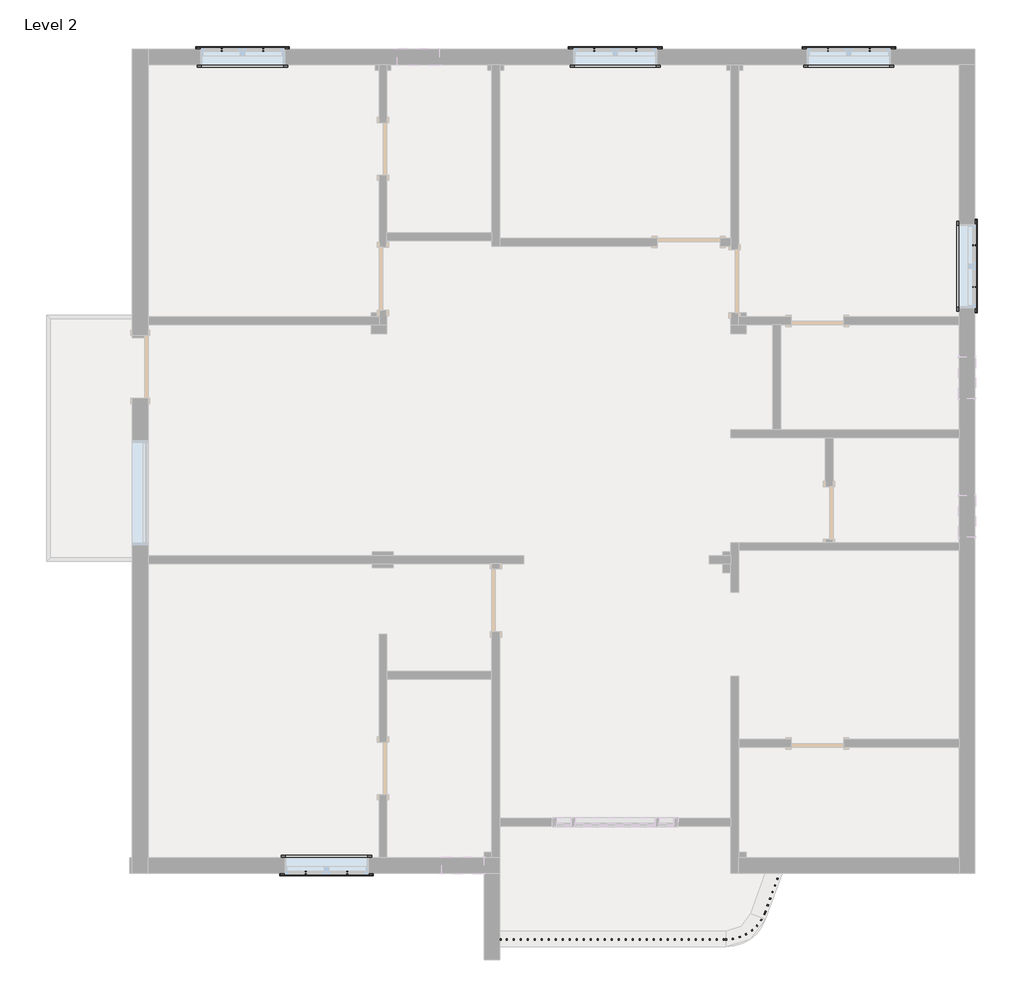
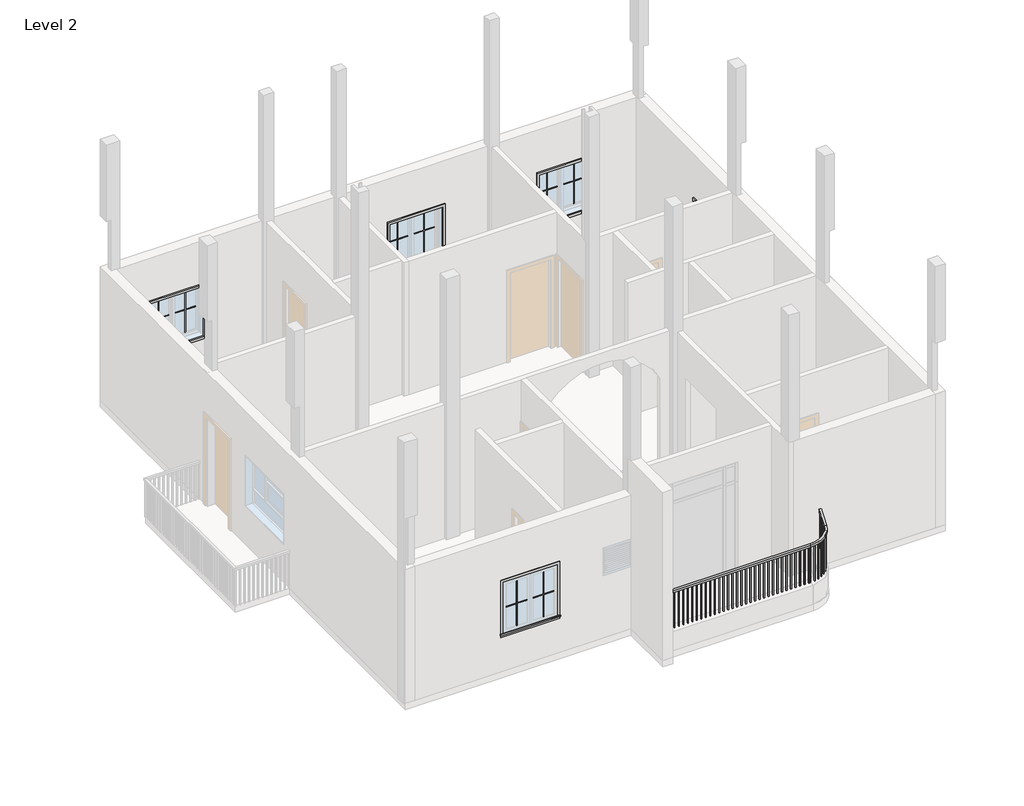
# One storey, part 4 of 4: 20 proxies, 1 railing.
"""IFC4 building model written with IfcOpenShell, lengths in millimetres."""

from ifc_helpers import new_model, si_unit, frame, origin, place, context, project, spatial, polyline, circle_curve, outline, extrude, transform, mapped, element, save
from ifc_brep_helpers import plane_surface, cylinder_surface, revolved_surface, advanced_brep
from components import muntin_pattern_2x2_muntin_pattern_2x2_4dfeb3f3, muntin_pattern_2x2_muntin_pattern_2x2_e852a7e4, trim_window_exterior_flat_with_sill_7cfdd449, trim_window_interior_flat_picture_frame_f1e0b15b

model = new_model("IFC4")

# Units and contexts
model_context = context("Model", 3, world=origin())
ifc_project = project(units=[si_unit("LENGTHUNIT", "METRE", prefix="MILLI")], contexts=[model_context])

# Site, building, storey
site = spatial("IfcSite", under=ifc_project)
building = spatial("IfcBuilding", under=site)
storey = spatial("IfcBuildingStorey", under=building, Name="Level 2", Elevation=3200.4)

# Proxies
placement = place(None, origin())
muntin_pattern_2x2_muntin_pattern_2x2_shape = muntin_pattern_2x2_muntin_pattern_2x2_4dfeb3f3(model_context)
element("IfcBuildingElementProxy", 1, Name="Muntin Pattern_2x2 : Muntin Pattern_2x2", ObjectType="Muntin Pattern_2x2 : Muntin Pattern_2x2", at=placement, inside=storey, context=model_context, shape_type="MappedRepresentation", body=[
    mapped(muntin_pattern_2x2_muntin_pattern_2x2_shape, transform((-13598.9803125, 13522.091018, 4184.65), x_axis=(1.0, 0.0, 0.0), y_axis=(0.0, 1.0, 0.0), z_axis=(0.0, 0.0, 1.0))),
])
element("IfcBuildingElementProxy", 2, Name="Muntin Pattern_2x2 : Muntin Pattern_2x2", ObjectType="Muntin Pattern_2x2 : Muntin Pattern_2x2", at=placement, inside=storey, context=model_context, shape_type="MappedRepresentation", body=[
    mapped(muntin_pattern_2x2_muntin_pattern_2x2_shape, transform((-8188.7803125, 13522.091018, 4184.65), x_axis=(1.0, 0.0, 0.0), y_axis=(0.0, 1.0, 0.0), z_axis=(0.0, 0.0, 1.0))),
])
element("IfcBuildingElementProxy", 3, Name="Muntin Pattern_2x2 : Muntin Pattern_2x2", ObjectType="Muntin Pattern_2x2 : Muntin Pattern_2x2", at=placement, inside=storey, context=model_context, shape_type="MappedRepresentation", body=[
    mapped(muntin_pattern_2x2_muntin_pattern_2x2_shape, transform((-4797.8803125, 13522.091018, 4184.65), x_axis=(1.0, 0.0, 0.0), y_axis=(0.0, 1.0, 0.0), z_axis=(0.0, 0.0, 1.0))),
])
element("IfcBuildingElementProxy", 4, Name="Muntin Pattern_2x2 : Muntin Pattern_2x2", ObjectType="Muntin Pattern_2x2 : Muntin Pattern_2x2", at=placement, inside=storey, context=model_context, shape_type="MappedRepresentation", body=[
    mapped(muntin_pattern_2x2_muntin_pattern_2x2_shape, transform((-2675.3928125, 10685.228518, 4184.65), x_axis=(0.0, -1.0, 0.0), y_axis=(1.0, 0.0, 0.0), z_axis=(0.0, 0.0, 1.0))),
])
element("IfcBuildingElementProxy", 5, Name="Muntin Pattern_2x2 : Muntin Pattern_2x2", ObjectType="Muntin Pattern_2x2 : Muntin Pattern_2x2", at=placement, inside=storey, context=model_context, shape_type="MappedRepresentation", body=[
    mapped(muntin_pattern_2x2_muntin_pattern_2x2_shape, transform((-11773.3553125, 1577.741018, 4184.65), x_axis=(-1.0, 0.0, 0.0), y_axis=(0.0, -1.0, 0.0), z_axis=(0.0, 0.0, 1.0))),
])
muntin_pattern_2x2_muntin_pattern_2x2_2_shape = muntin_pattern_2x2_muntin_pattern_2x2_e852a7e4(model_context)
element("IfcBuildingElementProxy", 6, Name="Muntin Pattern_2x2 : Muntin Pattern_2x2", ObjectType="Muntin Pattern_2x2 : Muntin Pattern_2x2", at=placement, inside=storey, context=model_context, shape_type="MappedRepresentation", body=[
    mapped(muntin_pattern_2x2_muntin_pattern_2x2_2_shape, transform((-12992.5553125, 13522.091018, 4184.65), x_axis=(-1.0, 0.0, 0.0), y_axis=(0.0, -1.0, 0.0), z_axis=(0.0, 0.0, 1.0))),
])
element("IfcBuildingElementProxy", 7, Name="Muntin Pattern_2x2 : Muntin Pattern_2x2", ObjectType="Muntin Pattern_2x2 : Muntin Pattern_2x2", at=placement, inside=storey, context=model_context, shape_type="MappedRepresentation", body=[
    mapped(muntin_pattern_2x2_muntin_pattern_2x2_2_shape, transform((-7582.3553125, 13522.091018, 4184.65), x_axis=(-1.0, 0.0, 0.0), y_axis=(0.0, -1.0, 0.0), z_axis=(0.0, 0.0, 1.0))),
])
element("IfcBuildingElementProxy", 8, Name="Muntin Pattern_2x2 : Muntin Pattern_2x2", ObjectType="Muntin Pattern_2x2 : Muntin Pattern_2x2", at=placement, inside=storey, context=model_context, shape_type="MappedRepresentation", body=[
    mapped(muntin_pattern_2x2_muntin_pattern_2x2_2_shape, transform((-4191.4553125, 13522.091018, 4184.65), x_axis=(-1.0, 0.0, 0.0), y_axis=(0.0, -1.0, 0.0), z_axis=(0.0, 0.0, 1.0))),
])
element("IfcBuildingElementProxy", 9, Name="Muntin Pattern_2x2 : Muntin Pattern_2x2", ObjectType="Muntin Pattern_2x2 : Muntin Pattern_2x2", at=placement, inside=storey, context=model_context, shape_type="MappedRepresentation", body=[
    mapped(muntin_pattern_2x2_muntin_pattern_2x2_2_shape, transform((-2675.3928125, 10078.803518, 4184.65), x_axis=(0.0, 1.0, 0.0), y_axis=(-1.0, 0.0, 0.0), z_axis=(0.0, 0.0, 1.0))),
])
element("IfcBuildingElementProxy", 10, Name="Muntin Pattern_2x2 : Muntin Pattern_2x2", ObjectType="Muntin Pattern_2x2 : Muntin Pattern_2x2", at=placement, inside=storey, context=model_context, shape_type="MappedRepresentation", body=[
    mapped(muntin_pattern_2x2_muntin_pattern_2x2_2_shape, transform((-12379.7803125, 1577.741018, 4184.65), x_axis=(1.0, 0.0, 0.0), y_axis=(0.0, 1.0, 0.0), z_axis=(0.0, 0.0, 1.0))),
])
trim_window_exterior_flat_with_sill_shape = trim_window_exterior_flat_with_sill_7cfdd449(model_context)
element("IfcBuildingElementProxy", 11, Name="Trim-Window-Exterior-Flat : with Sill", ObjectType="Trim-Window-Exterior-Flat : with Sill", at=placement, inside=storey, context=model_context, shape_type="MappedRepresentation", body=[
    mapped(trim_window_exterior_flat_with_sill_shape, transform((-13295.7678125, 13531.616018, 5334.0), x_axis=(-1.0, 0.0, 0.0), y_axis=(0.0, 0.0, 1.0), z_axis=(0.0, 1.0, 0.0))),
])
element("IfcBuildingElementProxy", 12, Name="Trim-Window-Exterior-Flat : with Sill", ObjectType="Trim-Window-Exterior-Flat : with Sill", at=placement, inside=storey, context=model_context, shape_type="MappedRepresentation", body=[
    mapped(trim_window_exterior_flat_with_sill_shape, transform((-7885.5678125, 13531.616018, 5334.0), x_axis=(-1.0, 0.0, 0.0), y_axis=(0.0, 0.0, 1.0), z_axis=(0.0, 1.0, 0.0))),
])
element("IfcBuildingElementProxy", 13, Name="Trim-Window-Exterior-Flat : with Sill", ObjectType="Trim-Window-Exterior-Flat : with Sill", at=placement, inside=storey, context=model_context, shape_type="MappedRepresentation", body=[
    mapped(trim_window_exterior_flat_with_sill_shape, transform((-4494.6678125, 13531.616018, 5334.0), x_axis=(-1.0, 0.0, 0.0), y_axis=(0.0, 0.0, 1.0), z_axis=(0.0, 1.0, 0.0))),
])
element("IfcBuildingElementProxy", 14, Name="Trim-Window-Exterior-Flat : with Sill", ObjectType="Trim-Window-Exterior-Flat : with Sill", at=placement, inside=storey, context=model_context, shape_type="MappedRepresentation", body=[
    mapped(trim_window_exterior_flat_with_sill_shape, transform((-2665.8678125, 10382.016018, 5334.0), x_axis=(0.0, 1.0, 0.0), y_axis=(0.0, 0.0, 1.0), z_axis=(1.0, 0.0, 0.0))),
])
element("IfcBuildingElementProxy", 15, Name="Trim-Window-Exterior-Flat : with Sill", ObjectType="Trim-Window-Exterior-Flat : with Sill", at=placement, inside=storey, context=model_context, shape_type="MappedRepresentation", body=[
    mapped(trim_window_exterior_flat_with_sill_shape, transform((-12076.5678125, 1568.216018, 5334.0), x_axis=(1.0, 0.0, 0.0), y_axis=(0.0, 0.0, 1.0), z_axis=(0.0, -1.0, 0.0))),
])
trim_window_interior_flat_picture_frame_shape = trim_window_interior_flat_picture_frame_f1e0b15b(model_context)
element("IfcBuildingElementProxy", 16, Name="Trim-Window-Interior-Flat : Picture Frame", ObjectType="Trim-Window-Interior-Flat : Picture Frame", at=placement, inside=storey, context=model_context, shape_type="MappedRepresentation", body=[
    mapped(trim_window_interior_flat_picture_frame_shape, transform((-13295.7678125, 13303.016018, 5334.0), x_axis=(1.0, 0.0, 0.0), y_axis=(0.0, 0.0, 1.0), z_axis=(0.0, -1.0, 0.0))),
])
element("IfcBuildingElementProxy", 17, Name="Trim-Window-Interior-Flat : Picture Frame", ObjectType="Trim-Window-Interior-Flat : Picture Frame", at=placement, inside=storey, context=model_context, shape_type="MappedRepresentation", body=[
    mapped(trim_window_interior_flat_picture_frame_shape, transform((-7885.5678125, 13303.016018, 5334.0), x_axis=(1.0, 0.0, 0.0), y_axis=(0.0, 0.0, 1.0), z_axis=(0.0, -1.0, 0.0))),
])
element("IfcBuildingElementProxy", 18, Name="Trim-Window-Interior-Flat : Picture Frame", ObjectType="Trim-Window-Interior-Flat : Picture Frame", at=placement, inside=storey, context=model_context, shape_type="MappedRepresentation", body=[
    mapped(trim_window_interior_flat_picture_frame_shape, transform((-4494.6678125, 13303.016018, 5334.0), x_axis=(1.0, 0.0, 0.0), y_axis=(0.0, 0.0, 1.0), z_axis=(0.0, -1.0, 0.0))),
])
element("IfcBuildingElementProxy", 19, Name="Trim-Window-Interior-Flat : Picture Frame", ObjectType="Trim-Window-Interior-Flat : Picture Frame", at=placement, inside=storey, context=model_context, shape_type="MappedRepresentation", body=[
    mapped(trim_window_interior_flat_picture_frame_shape, transform((-2894.4678125, 10382.016018, 5334.0), x_axis=(0.0, -1.0, 0.0), y_axis=(0.0, 0.0, 1.0), z_axis=(-1.0, 0.0, 0.0))),
])
element("IfcBuildingElementProxy", 20, Name="Trim-Window-Interior-Flat : Picture Frame", ObjectType="Trim-Window-Interior-Flat : Picture Frame", at=placement, inside=storey, context=model_context, shape_type="MappedRepresentation", body=[
    mapped(trim_window_interior_flat_picture_frame_shape, transform((-12076.5678125, 1796.816018, 5334.0), x_axis=(-1.0, 0.0, 0.0), y_axis=(0.0, 0.0, 1.0), z_axis=(0.0, 1.0, 0.0))),
])

# Railing
element("IfcRailing", 21, ObjectType="Handrail - Rectangular", at=placement, inside=storey, context=model_context, shape_type="SolidModel", body=[
    advanced_brep(
    [(-9561.9678125, 634.766018, 4572.0), (-9561.9678125, 634.766018, 4521.2), (-9561.9678125, 583.966018, 4521.2), (-9561.9678125, 583.966018, 4572.0), (-6278.443289, 634.766018, 4572.0), (-6278.443289, 634.766018, 4521.2), (-6278.443289, 583.966018, 4521.2), (-6278.443289, 583.966018, 4572.0), (-5729.4748599, 1019.1578503, 4521.2), (-5729.4748599, 1019.1578503, 4572.0), (-5681.7384748, 1001.783227, 4521.2), (-5681.7384748, 1001.783227, 4572.0), (-5487.1815204, 1684.8533296, 4572.0), (-5439.4451352, 1667.4787064, 4572.0), (-5439.4451352, 1667.4787064, 4521.2), (-5487.1815204, 1684.8533296, 4521.2)],
    [
        (0, 1),
        (1, 2),
        (2, 3),
        (3, 0),
        (0, 4),
        (4, 5),
        (5, 1),
        (5, 6),
        (6, 2),
        (6, 7),
        (7, 3),
        (7, 4),
        (8, 5, circle_curve(frame((-6278.443289, 1218.966018, 4521.2), z_axis=(0.0, 0.0, -1.0), x_axis=(0.0, -1.0, 0.0)), 584.2)),
        (4, 9, circle_curve(frame((-6278.443289, 1218.966018, 4572.0), z_axis=(0.0, 0.0, 1.0), x_axis=(0.0, -1.0, 0.0)), 584.2)),
        (9, 8),
        (10, 6, circle_curve(frame((-6278.443289, 1218.966018, 4521.2), z_axis=(0.0, 0.0, -1.0), x_axis=(0.0, -1.0, 0.0)), 635.0)),
        (8, 10),
        (11, 7, circle_curve(frame((-6278.443289, 1218.966018, 4572.0), z_axis=(0.0, 0.0, -1.0), x_axis=(0.0, -1.0, 0.0)), 635.0)),
        (10, 11),
        (11, 9),
        (12, 13),
        (13, 14),
        (14, 15),
        (15, 12),
        (9, 12),
        (15, 8),
        (14, 10),
        (13, 11),
    ],
    [
        plane_surface(frame((-9561.9678125, 609.366018, 4572.0), z_axis=(-1.0, 0.0, 0.0), x_axis=(0.0, 1.0, 0.0))),
        plane_surface(frame((-9561.9678125, 634.766018, 4572.0), z_axis=(0.0, 1.0, 0.0), x_axis=(1.0, 0.0, 0.0))),
        plane_surface(frame((-9561.9678125, 634.766018, 4521.2), z_axis=(0.0, 0.0, -1.0), x_axis=(1.0, 0.0, 0.0))),
        plane_surface(frame((-9561.9678125, 583.966018, 4521.2), z_axis=(0.0, -1.0, 0.0), x_axis=(1.0, 0.0, 0.0))),
        plane_surface(frame((-9561.9678125, 583.966018, 4572.0), z_axis=(0.0, 0.0, 1.0), x_axis=(1.0, 0.0, 0.0))),
        revolved_surface(polyline([(-6278.443289, 634.766018, 4572.0), (-6278.443289, 634.766018, 4521.2)]), (-6278.443289, 1218.966018, 4572.0), (0.0, 0.0, 1.0)),
        plane_surface(frame((-6278.443289, 1218.966018, 4521.2), z_axis=(0.0, 0.0, -1.0), x_axis=(0.0, -1.0, 0.0))),
        cylinder_surface(frame((-6278.443289, 1218.966018, 4572.0), z_axis=(0.0, 0.0, 1.0), x_axis=(0.0, -1.0, 0.0)), 635.0),
        plane_surface(frame((-6278.443289, 1218.966018, 4572.0), z_axis=(0.0, 0.0, 1.0), x_axis=(0.0, -1.0, 0.0))),
        plane_surface(frame((-5463.3133278, 1676.166018, 4572.0), z_axis=(0.3420201433256705, 0.9396926207859078, 0.0), x_axis=(0.9396926207859078, -0.3420201433256705, 0.0))),
        plane_surface(frame((-5729.4748599, 1019.1578503, 4572.0), z_axis=(-0.9396926207859078, 0.3420201433256704, 0.0), x_axis=(0.3420201433256704, 0.9396926207859078, 0.0))),
        plane_surface(frame((-5729.4748599, 1019.1578503, 4521.2), z_axis=(0.0, 0.0, -1.0), x_axis=(0.3420201433256704, 0.9396926207859078, 0.0))),
        plane_surface(frame((-5681.7384748, 1001.783227, 4521.2), z_axis=(0.9396926207859079, -0.3420201433256703, 0.0), x_axis=(0.3420201433256703, 0.9396926207859079, 0.0))),
        plane_surface(frame((-5681.7384748, 1001.783227, 4572.0), z_axis=(0.0, 0.0, 1.0), x_axis=(0.3420201433256703, 0.9396926207859079, 0.0))),
    ],
    [
        (0, [[1, 2, 3, 4]]),
        (1, [[-1, 5, 6, 7]]),
        (2, [[-2, -7, 8, 9]]),
        (3, [[-3, -9, 10, 11]]),
        (4, [[-4, -11, 12, -5]]),
        (5, [[13, -6, 14, 15]]),
        (6, [[16, -8, -13, 17]]),
        (7, [[18, -10, -16, 19]]),
        (8, [[-14, -12, -18, 20]]),
        (9, [[21, 22, 23, 24]]),
        (10, [[-15, 25, -24, 26]]),
        (11, [[-17, -26, -23, 27]]),
        (12, [[-19, -27, -22, 28]]),
        (13, [[-20, -28, -21, -25]]),
    ],
),
    extrude(outline(polyline([(-5491.4183577, 1571.0988462), (-5509.3195021, 1577.6143299), (-5502.8040184, 1595.5154743), (-5484.9028739, 1588.9999906), (-5491.4183577, 1571.0988462)])), frame((0.0, 0.0, 3657.6), z_axis=(0.0, 0.0, 1.0), x_axis=(1.0, 0.0, 0.0)), (0.0, 0.0, 1.0), 863.6),
    extrude(outline(polyline([(-5526.1676042, 1475.6260759), (-5544.0687486, 1482.1415596), (-5537.5532649, 1500.0427041), (-5519.6521205, 1493.5272203), (-5526.1676042, 1475.6260759)])), frame((0.0, 0.0, 3657.6), z_axis=(0.0, 0.0, 1.0), x_axis=(1.0, 0.0, 0.0)), (0.0, 0.0, 1.0), 863.6),
    extrude(outline(polyline([(-5560.9168508, 1380.1533056), (-5578.8179952, 1386.6687894), (-5572.3025115, 1404.5699338), (-5554.4013671, 1398.0544501), (-5560.9168508, 1380.1533056)])), frame((0.0, 0.0, 3657.6), z_axis=(0.0, 0.0, 1.0), x_axis=(1.0, 0.0, 0.0)), (0.0, 0.0, 1.0), 863.6),
    extrude(outline(polyline([(-5595.6660973, 1284.6805354), (-5613.5672418, 1291.1960191), (-5607.051758, 1309.0971635), (-5589.1506136, 1302.5816798), (-5595.6660973, 1284.6805354)])), frame((0.0, 0.0, 3657.6), z_axis=(0.0, 0.0, 1.0), x_axis=(1.0, 0.0, 0.0)), (0.0, 0.0, 1.0), 863.6),
    extrude(outline(polyline([(-5630.4153439, 1189.2077651), (-5648.3164883, 1195.7232488), (-5641.8010046, 1213.6243932), (-5623.8998602, 1207.1089095), (-5630.4153439, 1189.2077651)])), frame((0.0, 0.0, 3657.6), z_axis=(0.0, 0.0, 1.0), x_axis=(1.0, 0.0, 0.0)), (0.0, 0.0, 1.0), 863.6),
    extrude(outline(polyline([(-5665.1645905, 1093.7349948), (-5683.0657349, 1100.2504785), (-5676.5502512, 1118.151623), (-5658.6491067, 1111.6361392), (-5665.1645905, 1093.7349948)])), frame((0.0, 0.0, 3657.6), z_axis=(0.0, 0.0, 1.0), x_axis=(1.0, 0.0, 0.0)), (0.0, 0.0, 1.0), 863.6),
    extrude(outline(polyline([(-5712.9373242, 966.7567894), (-5730.452751, 974.2476053), (-5722.9619352, 991.7630322), (-5705.4465083, 984.2722163), (-5712.9373242, 966.7567894)])), frame((0.0, 0.0, 3657.6), z_axis=(0.0, 0.0, 1.0), x_axis=(1.0, 0.0, 0.0)), (0.0, 0.0, 1.0), 863.6),
    extrude(outline(polyline([(-5762.613945, 876.4363417), (-5778.6439673, 886.7291007), (-5768.3512083, 902.7591229), (-5752.3211861, 892.466364), (-5762.613945, 876.4363417)])), frame((0.0, 0.0, 3657.6), z_axis=(0.0, 0.0, 1.0), x_axis=(1.0, 0.0, 0.0)), (0.0, 0.0, 1.0), 863.6),
    extrude(outline(polyline([(-5826.5860214, 795.6086028), (-5840.6863905, 808.4180561), (-5827.8769372, 822.5184252), (-5813.7765681, 809.7089719), (-5826.5860214, 795.6086028)])), frame((0.0, 0.0, 3657.6), z_axis=(0.0, 0.0, 1.0), x_axis=(1.0, 0.0, 0.0)), (0.0, 0.0, 1.0), 863.6),
    extrude(outline(polyline([(-5903.0806608, 726.5135953), (-5914.8606056, 741.4847476), (-5899.8894533, 753.2646924), (-5888.1095085, 738.29354), (-5903.0806608, 726.5135953)])), frame((0.0, 0.0, 3657.6), z_axis=(0.0, 0.0, 1.0), x_axis=(1.0, 0.0, 0.0)), (0.0, 0.0, 1.0), 863.6),
    extrude(outline(polyline([(-5989.9779263, 671.0661861), (-5999.1109828, 687.7841339), (-5982.393035, 696.9171904), (-5973.2599785, 680.1992426), (-5989.9779263, 671.0661861)])), frame((0.0, 0.0, 3657.6), z_axis=(0.0, 0.0, 1.0), x_axis=(1.0, 0.0, 0.0)), (0.0, 0.0, 1.0), 863.6),
    extrude(outline(polyline([(-6084.8695873, 630.8030191), (-6091.1026462, 648.8044489), (-6073.1012164, 655.0375079), (-6066.8681574, 637.0360781), (-6084.8695873, 630.8030191)])), frame((0.0, 0.0, 3657.6), z_axis=(0.0, 0.0, 1.0), x_axis=(1.0, 0.0, 0.0)), (0.0, 0.0, 1.0), 863.6),
    extrude(outline(polyline([(-6185.1258601, 606.8399291), (-6188.2861815, 625.6259576), (-6169.5001529, 628.786279), (-6166.3398316, 610.0002504), (-6185.1258601, 606.8399291)])), frame((0.0, 0.0, 3657.6), z_axis=(0.0, 0.0, 1.0), x_axis=(1.0, 0.0, 0.0)), (0.0, 0.0, 1.0), 863.6),
    extrude(outline(polyline([(-6320.2928125, 599.841018), (-6320.2928125, 618.891018), (-6301.2428125, 618.891018), (-6301.2428125, 599.841018), (-6320.2928125, 599.841018)])), frame((0.0, 0.0, 3657.6), z_axis=(0.0, 0.0, 1.0), x_axis=(1.0, 0.0, 0.0)), (0.0, 0.0, 1.0), 863.6),
    extrude(outline(polyline([(-6421.8928125, 599.841018), (-6421.8928125, 618.891018), (-6402.8428125, 618.891018), (-6402.8428125, 599.841018), (-6421.8928125, 599.841018)])), frame((0.0, 0.0, 3657.6), z_axis=(0.0, 0.0, 1.0), x_axis=(1.0, 0.0, 0.0)), (0.0, 0.0, 1.0), 863.6),
    extrude(outline(polyline([(-6523.4928125, 599.841018), (-6523.4928125, 618.891018), (-6504.4428125, 618.891018), (-6504.4428125, 599.841018), (-6523.4928125, 599.841018)])), frame((0.0, 0.0, 3657.6), z_axis=(0.0, 0.0, 1.0), x_axis=(1.0, 0.0, 0.0)), (0.0, 0.0, 1.0), 863.6),
    extrude(outline(polyline([(-6625.0928125, 599.841018), (-6625.0928125, 618.891018), (-6606.0428125, 618.891018), (-6606.0428125, 599.841018), (-6625.0928125, 599.841018)])), frame((0.0, 0.0, 3657.6), z_axis=(0.0, 0.0, 1.0), x_axis=(1.0, 0.0, 0.0)), (0.0, 0.0, 1.0), 863.6),
    extrude(outline(polyline([(-6726.6928125, 599.841018), (-6726.6928125, 618.891018), (-6707.6428125, 618.891018), (-6707.6428125, 599.841018), (-6726.6928125, 599.841018)])), frame((0.0, 0.0, 3657.6), z_axis=(0.0, 0.0, 1.0), x_axis=(1.0, 0.0, 0.0)), (0.0, 0.0, 1.0), 863.6),
    extrude(outline(polyline([(-6828.2928125, 599.841018), (-6828.2928125, 618.891018), (-6809.2428125, 618.891018), (-6809.2428125, 599.841018), (-6828.2928125, 599.841018)])), frame((0.0, 0.0, 3657.6), z_axis=(0.0, 0.0, 1.0), x_axis=(1.0, 0.0, 0.0)), (0.0, 0.0, 1.0), 863.6),
    extrude(outline(polyline([(-6929.8928125, 599.841018), (-6929.8928125, 618.891018), (-6910.8428125, 618.891018), (-6910.8428125, 599.841018), (-6929.8928125, 599.841018)])), frame((0.0, 0.0, 3657.6), z_axis=(0.0, 0.0, 1.0), x_axis=(1.0, 0.0, 0.0)), (0.0, 0.0, 1.0), 863.6),
    extrude(outline(polyline([(-7031.4928125, 599.841018), (-7031.4928125, 618.891018), (-7012.4428125, 618.891018), (-7012.4428125, 599.841018), (-7031.4928125, 599.841018)])), frame((0.0, 0.0, 3657.6), z_axis=(0.0, 0.0, 1.0), x_axis=(1.0, 0.0, 0.0)), (0.0, 0.0, 1.0), 863.6),
    extrude(outline(polyline([(-7133.0928125, 599.841018), (-7133.0928125, 618.891018), (-7114.0428125, 618.891018), (-7114.0428125, 599.841018), (-7133.0928125, 599.841018)])), frame((0.0, 0.0, 3657.6), z_axis=(0.0, 0.0, 1.0), x_axis=(1.0, 0.0, 0.0)), (0.0, 0.0, 1.0), 863.6),
    extrude(outline(polyline([(-7234.6928125, 599.841018), (-7234.6928125, 618.891018), (-7215.6428125, 618.891018), (-7215.6428125, 599.841018), (-7234.6928125, 599.841018)])), frame((0.0, 0.0, 3657.6), z_axis=(0.0, 0.0, 1.0), x_axis=(1.0, 0.0, 0.0)), (0.0, 0.0, 1.0), 863.6),
    extrude(outline(polyline([(-7336.2928125, 599.841018), (-7336.2928125, 618.891018), (-7317.2428125, 618.891018), (-7317.2428125, 599.841018), (-7336.2928125, 599.841018)])), frame((0.0, 0.0, 3657.6), z_axis=(0.0, 0.0, 1.0), x_axis=(1.0, 0.0, 0.0)), (0.0, 0.0, 1.0), 863.6),
    extrude(outline(polyline([(-7437.8928125, 599.841018), (-7437.8928125, 618.891018), (-7418.8428125, 618.891018), (-7418.8428125, 599.841018), (-7437.8928125, 599.841018)])), frame((0.0, 0.0, 3657.6), z_axis=(0.0, 0.0, 1.0), x_axis=(1.0, 0.0, 0.0)), (0.0, 0.0, 1.0), 863.6),
    extrude(outline(polyline([(-7539.4928125, 599.841018), (-7539.4928125, 618.891018), (-7520.4428125, 618.891018), (-7520.4428125, 599.841018), (-7539.4928125, 599.841018)])), frame((0.0, 0.0, 3657.6), z_axis=(0.0, 0.0, 1.0), x_axis=(1.0, 0.0, 0.0)), (0.0, 0.0, 1.0), 863.6),
    extrude(outline(polyline([(-7641.0928125, 599.841018), (-7641.0928125, 618.891018), (-7622.0428125, 618.891018), (-7622.0428125, 599.841018), (-7641.0928125, 599.841018)])), frame((0.0, 0.0, 3657.6), z_axis=(0.0, 0.0, 1.0), x_axis=(1.0, 0.0, 0.0)), (0.0, 0.0, 1.0), 863.6),
    extrude(outline(polyline([(-7742.6928125, 599.841018), (-7742.6928125, 618.891018), (-7723.6428125, 618.891018), (-7723.6428125, 599.841018), (-7742.6928125, 599.841018)])), frame((0.0, 0.0, 3657.6), z_axis=(0.0, 0.0, 1.0), x_axis=(1.0, 0.0, 0.0)), (0.0, 0.0, 1.0), 863.6),
    extrude(outline(polyline([(-7844.2928125, 599.841018), (-7844.2928125, 618.891018), (-7825.2428125, 618.891018), (-7825.2428125, 599.841018), (-7844.2928125, 599.841018)])), frame((0.0, 0.0, 3657.6), z_axis=(0.0, 0.0, 1.0), x_axis=(1.0, 0.0, 0.0)), (0.0, 0.0, 1.0), 863.6),
    extrude(outline(polyline([(-7945.8928125, 599.841018), (-7945.8928125, 618.891018), (-7926.8428125, 618.891018), (-7926.8428125, 599.841018), (-7945.8928125, 599.841018)])), frame((0.0, 0.0, 3657.6), z_axis=(0.0, 0.0, 1.0), x_axis=(1.0, 0.0, 0.0)), (0.0, 0.0, 1.0), 863.6),
    extrude(outline(polyline([(-8047.4928125, 599.841018), (-8047.4928125, 618.891018), (-8028.4428125, 618.891018), (-8028.4428125, 599.841018), (-8047.4928125, 599.841018)])), frame((0.0, 0.0, 3657.6), z_axis=(0.0, 0.0, 1.0), x_axis=(1.0, 0.0, 0.0)), (0.0, 0.0, 1.0), 863.6),
    extrude(outline(polyline([(-8149.0928125, 599.841018), (-8149.0928125, 618.891018), (-8130.0428125, 618.891018), (-8130.0428125, 599.841018), (-8149.0928125, 599.841018)])), frame((0.0, 0.0, 3657.6), z_axis=(0.0, 0.0, 1.0), x_axis=(1.0, 0.0, 0.0)), (0.0, 0.0, 1.0), 863.6),
    extrude(outline(polyline([(-8250.6928125, 599.841018), (-8250.6928125, 618.891018), (-8231.6428125, 618.891018), (-8231.6428125, 599.841018), (-8250.6928125, 599.841018)])), frame((0.0, 0.0, 3657.6), z_axis=(0.0, 0.0, 1.0), x_axis=(1.0, 0.0, 0.0)), (0.0, 0.0, 1.0), 863.6),
    extrude(outline(polyline([(-8352.2928125, 599.841018), (-8352.2928125, 618.891018), (-8333.2428125, 618.891018), (-8333.2428125, 599.841018), (-8352.2928125, 599.841018)])), frame((0.0, 0.0, 3657.6), z_axis=(0.0, 0.0, 1.0), x_axis=(1.0, 0.0, 0.0)), (0.0, 0.0, 1.0), 863.6),
    extrude(outline(polyline([(-8453.8928125, 599.841018), (-8453.8928125, 618.891018), (-8434.8428125, 618.891018), (-8434.8428125, 599.841018), (-8453.8928125, 599.841018)])), frame((0.0, 0.0, 3657.6), z_axis=(0.0, 0.0, 1.0), x_axis=(1.0, 0.0, 0.0)), (0.0, 0.0, 1.0), 863.6),
    extrude(outline(polyline([(-8555.4928125, 599.841018), (-8555.4928125, 618.891018), (-8536.4428125, 618.891018), (-8536.4428125, 599.841018), (-8555.4928125, 599.841018)])), frame((0.0, 0.0, 3657.6), z_axis=(0.0, 0.0, 1.0), x_axis=(1.0, 0.0, 0.0)), (0.0, 0.0, 1.0), 863.6),
    extrude(outline(polyline([(-8657.0928125, 599.841018), (-8657.0928125, 618.891018), (-8638.0428125, 618.891018), (-8638.0428125, 599.841018), (-8657.0928125, 599.841018)])), frame((0.0, 0.0, 3657.6), z_axis=(0.0, 0.0, 1.0), x_axis=(1.0, 0.0, 0.0)), (0.0, 0.0, 1.0), 863.6),
    extrude(outline(polyline([(-8758.6928125, 599.841018), (-8758.6928125, 618.891018), (-8739.6428125, 618.891018), (-8739.6428125, 599.841018), (-8758.6928125, 599.841018)])), frame((0.0, 0.0, 3657.6), z_axis=(0.0, 0.0, 1.0), x_axis=(1.0, 0.0, 0.0)), (0.0, 0.0, 1.0), 863.6),
    extrude(outline(polyline([(-8860.2928125, 599.841018), (-8860.2928125, 618.891018), (-8841.2428125, 618.891018), (-8841.2428125, 599.841018), (-8860.2928125, 599.841018)])), frame((0.0, 0.0, 3657.6), z_axis=(0.0, 0.0, 1.0), x_axis=(1.0, 0.0, 0.0)), (0.0, 0.0, 1.0), 863.6),
    extrude(outline(polyline([(-8961.8928125, 599.841018), (-8961.8928125, 618.891018), (-8942.8428125, 618.891018), (-8942.8428125, 599.841018), (-8961.8928125, 599.841018)])), frame((0.0, 0.0, 3657.6), z_axis=(0.0, 0.0, 1.0), x_axis=(1.0, 0.0, 0.0)), (0.0, 0.0, 1.0), 863.6),
    extrude(outline(polyline([(-9063.4928125, 599.841018), (-9063.4928125, 618.891018), (-9044.4428125, 618.891018), (-9044.4428125, 599.841018), (-9063.4928125, 599.841018)])), frame((0.0, 0.0, 3657.6), z_axis=(0.0, 0.0, 1.0), x_axis=(1.0, 0.0, 0.0)), (0.0, 0.0, 1.0), 863.6),
    extrude(outline(polyline([(-9165.0928125, 599.841018), (-9165.0928125, 618.891018), (-9146.0428125, 618.891018), (-9146.0428125, 599.841018), (-9165.0928125, 599.841018)])), frame((0.0, 0.0, 3657.6), z_axis=(0.0, 0.0, 1.0), x_axis=(1.0, 0.0, 0.0)), (0.0, 0.0, 1.0), 863.6),
    extrude(outline(polyline([(-9266.6928125, 599.841018), (-9266.6928125, 618.891018), (-9247.6428125, 618.891018), (-9247.6428125, 599.841018), (-9266.6928125, 599.841018)])), frame((0.0, 0.0, 3657.6), z_axis=(0.0, 0.0, 1.0), x_axis=(1.0, 0.0, 0.0)), (0.0, 0.0, 1.0), 863.6),
    extrude(outline(polyline([(-9368.2928125, 599.841018), (-9368.2928125, 618.891018), (-9349.2428125, 618.891018), (-9349.2428125, 599.841018), (-9368.2928125, 599.841018)])), frame((0.0, 0.0, 3657.6), z_axis=(0.0, 0.0, 1.0), x_axis=(1.0, 0.0, 0.0)), (0.0, 0.0, 1.0), 863.6),
    extrude(outline(polyline([(-9469.8928125, 599.841018), (-9469.8928125, 618.891018), (-9450.8428125, 618.891018), (-9450.8428125, 599.841018), (-9469.8928125, 599.841018)])), frame((0.0, 0.0, 3657.6), z_axis=(0.0, 0.0, 1.0), x_axis=(1.0, 0.0, 0.0)), (0.0, 0.0, 1.0), 863.6),
    extrude(outline(polyline([(-5699.913837, 998.2622245), (-5717.8149815, 1004.7777083), (-5711.2994977, 1022.6788527), (-5693.3983533, 1016.163369), (-5699.913837, 998.2622245)])), frame((0.0, 0.0, 3657.6), z_axis=(0.0, 0.0, 1.0), x_axis=(1.0, 0.0, 0.0)), (0.0, 0.0, 1.0), 863.6),
    extrude(outline(polyline([(-6287.968289, 599.841018), (-6287.968289, 618.891018), (-6268.918289, 618.891018), (-6268.918289, 599.841018), (-6287.968289, 599.841018)])), frame((0.0, 0.0, 3657.6), z_axis=(0.0, 0.0, 1.0), x_axis=(1.0, 0.0, 0.0)), (0.0, 0.0, 1.0), 863.6),
    extrude(outline(polyline([(-5460.8782393, 1655.0071317), (-5478.7793837, 1661.5226154), (-5472.2639, 1679.4237599), (-5454.3627556, 1672.9082761), (-5460.8782393, 1655.0071317)])), frame((0.0, 0.0, 3657.6), z_axis=(0.0, 0.0, 1.0), x_axis=(1.0, 0.0, 0.0)), (0.0, 0.0, 1.0), 863.6),
    extrude(outline(polyline([(-9561.9678125, 599.841018), (-9561.9678125, 618.891018), (-9542.9178125, 618.891018), (-9542.9178125, 599.841018), (-9561.9678125, 599.841018)])), frame((0.0, 0.0, 3657.6), z_axis=(0.0, 0.0, 1.0), x_axis=(1.0, 0.0, 0.0)), (0.0, 0.0, 1.0), 863.6),
])

save(model, "model.ifc")

# Revit data of these elements
# Type "Muntin Pattern_2x2 : Muntin Pattern_2x2"
#   Width [instance default] = 4' - 0"
#   Thickness = 0' - 0 1/2"
#   Height [instance default] = 4' - 0"
#   Distance = 0' - 0 3/4"
#   Interior Material [instance default] = none
#   Exterior Material [instance default] = none
#   Default Elevation = 0
# Type "Trim-Window-Exterior-Flat : with Sill"
#   Trim Width = 0' - 2 1/4"
#   Trim Thickness_Picture Frame = 0' - 1 1/4"
#   Trim Thickness_with Sill = 0' - 0 3/4"
#   Sill Thickness = 0' - 1 1/4"
#   Opening Width [instance default] = 2' - 0"
#   Opening Height [instance default] = 3' - 0"
#   Default Elevation = 4' - 0"
#   Sill = yes
#   Picture Frame = no
#   Trim Material [instance default] = none
# Type "Trim-Window-Interior-Flat : Picture Frame"
#   Trim Thickness_Picture Frame = 0' - 1 1/4"
#   Trim Width = 0' - 2 1/4"
#   Trim Thickness_with Sill = 0' - 0 3/4"
#   Sill Thickness = 0' - 1 1/4"
#   Opening Width [instance default] = 2' - 0"
#   Opening Height [instance default] = 3' - 0"
#   Default Elevation = 4' - 0"
#   Sill = no
#   Picture Frame = yes
#   Trim Material [instance default] = none
# Type "Handrail - Rectangular"
#   Assembly Code = "C2010400"
#   built-in parameter 1008612 = 0.0416667 (stored number, unit not read)
#   built-in parameter 1008611 = 0.0416667 (stored number, unit not read)
#   built-in parameter 1008609 = 0.333333 (stored number, unit not read)
#   built-in parameter 1008604 = 0.166667 (stored number, unit not read)
#   built-in parameter 1008603 = 0.166667 (stored number, unit not read)
#   Railing Height = 3' - 0"
#   built-in parameter 1008630 = 2
#   built-in parameter 1008610 = 2
#   built-in parameter 1008618 = Baluster - Square : 3/4"
# Elements 1, 2, 3, 4, 5, 6, 7, 8, 9, 10 (IfcBuildingElementProxy, "Muntin Pattern_2x2 : Muntin Pattern_2x2")
#   Width = 1' - 6 5/8"
#   Height = 3' - 6 1/2"
#   Interior Material = Wood - Stained
#   Exterior Material = Clad - White
#   Phase Created = New Construction
#   Materials on its faces: "Clad - White", "Wood - Stained"
# Elements 11, 12, 13, 14, 15 (IfcBuildingElementProxy, "Trim-Window-Exterior-Flat : with Sill")
#   Opening Width = 4' - 0"
#   Opening Height = 4' - 0"
#   Trim Material = Clad - White
#   Phase Created = New Construction
#   Materials on its faces: "Clad - White"
# Elements 16, 17, 18, 19, 20 (IfcBuildingElementProxy, "Trim-Window-Interior-Flat : Picture Frame")
#   Opening Width = 4' - 0"
#   Opening Height = 4' - 0"
#   Trim Material = Wood - Stained
#   Phase Created = New Construction
#   Materials on its faces: "Wood - Stained"
# Element 21 (IfcRailing, "Handrail - Rectangular")
#   built-in parameter 1008621 = 1.5 (stored number, unit not read)
#   Phase Created = New Construction
# Materials
#   "Clad - White": class "Wood", colour RGB 242 242 238, transparency 0, Cost = 0
#   "Wood - Stained": class "Wood", colour RGB 224 178 126, transparency 0, Cost = 0
